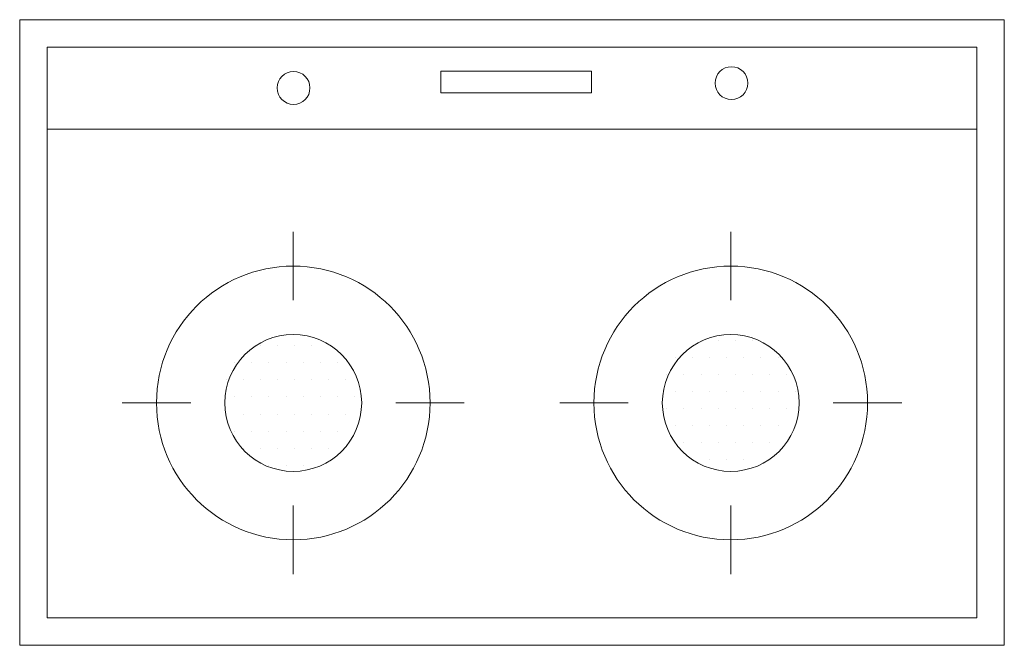
# Model space of a CAD drawing. Units: inches. Extents: x 205 to 1667, y -23 to 828.
# Tile 10 of 10: x 1560 to 1667, y 401 to 469. Entities that reach past the tile are written whole.
import ezdxf

# ---------------------------------------------------------------- set-up
doc = ezdxf.new("R2010")
doc.units = ezdxf.units.IN
doc.header["$MEASUREMENT"] = 0
doc.layers.add('A-EQPM', color=8, linetype='Continuous', lineweight=18)

# ---------------------------------------------------------------- blocks, each defined once
blk = doc.blocks.new('A$C475E21CF')
for p, q in [((0, 444.49), (0, 0)), ((0, 444.49), (699.92, 444.49)), ((699.92, 444.49), (699.92, 0)), ((19.45, 425.05), (19.45, 19.45)), ((19.45, 425.05), (680.48, 425.05)), ((680.48, 425.05), (680.48, 19.45)), ((194.48, 393.86), (194.48, 345.24)), ((505.44, 393.86), (505.44, 345.24)), ((498.43, 316.63), (498.43, 316.63)), ((510.58, 316.63), (510.58, 316.63)), ((522.74, 316.63), (522.74, 316.63)), ((185.17, 312.7), (185.17, 312.7)), ((197.32, 312.7), (197.32, 312.7)), ((209.48, 312.7), (209.48, 312.7)), ((480.19, 304.48), (480.19, 304.48)), ((492.35, 304.48), (492.35, 304.48)), ((504.5, 304.48), (504.5, 304.48)), ((516.66, 304.48), (516.66, 304.48)), ((528.81, 304.48), (528.81, 304.48)), ((540.97, 304.48), (540.97, 304.48)), ((166.94, 300.55), (166.94, 300.55)), ((179.09, 300.55), (179.09, 300.55)), ((191.25, 300.55), (191.25, 300.55)), ((203.4, 300.55), (203.4, 300.55)), ((215.56, 300.55), (215.56, 300.55)), ((227.71, 300.55), (227.71, 300.55)), ((160.86, 288.39), (160.86, 288.39)), ((173.01, 288.39), (173.01, 288.39)), ((185.17, 288.39), (185.17, 288.39)), ((197.32, 288.39), (197.32, 288.39)), ((209.48, 288.39), (209.48, 288.39)), ((221.63, 288.39), (221.63, 288.39)), ((233.79, 288.39), (233.79, 288.39)), ((474.12, 292.32), (474.12, 292.32)), ((486.27, 292.32), (486.27, 292.32)), ((498.43, 292.32), (498.43, 292.32)), ((510.58, 292.32), (510.58, 292.32)), ((522.74, 292.32), (522.74, 292.32)), ((534.89, 292.32), (534.89, 292.32)), ((547.05, 292.32), (547.05, 292.32)), ((468.04, 280.17), (468.04, 280.17)), ((480.19, 280.17), (480.19, 280.17)), ((492.35, 280.17), (492.35, 280.17)), ((504.5, 280.17), (504.5, 280.17)), ((516.66, 280.17), (516.66, 280.17)), ((528.81, 280.17), (528.81, 280.17)), ((540.97, 280.17), (540.97, 280.17)), ((553.12, 280.17), (553.12, 280.17)), ((154.78, 276.24), (154.78, 276.24)), ((166.94, 276.24), (166.94, 276.24)), ((179.09, 276.24), (179.09, 276.24)), ((191.25, 276.24), (191.25, 276.24)), ((203.4, 276.24), (203.4, 276.24)), ((215.56, 276.24), (215.56, 276.24)), ((227.71, 276.24), (227.71, 276.24)), ((239.87, 276.24), (239.87, 276.24)), ((72.93, 272.31), (121.55, 272.31)), ((267.41, 272.31), (316.03, 272.31)), ((383.89, 272.31), (432.51, 272.31)), ((461.96, 268.01), (461.96, 268.01)), ((474.12, 268.01), (474.12, 268.01)), ((486.27, 268.01), (486.27, 268.01)), ((498.43, 268.01), (498.43, 268.01)), ((510.58, 268.01), (510.58, 268.01)), ((522.74, 268.01), (522.74, 268.01)), ((534.89, 268.01), (534.89, 268.01)), ((547.05, 268.01), (547.05, 268.01)), ((578.37, 272.31), (626.99, 272.31)), ((148.7, 264.08), (148.7, 264.08)), ((160.86, 264.08), (160.86, 264.08)), ((173.01, 264.08), (173.01, 264.08)), ((185.17, 264.08), (185.17, 264.08)), ((197.32, 264.08), (197.32, 264.08)), ((209.48, 264.08), (209.48, 264.08)), ((221.63, 264.08), (221.63, 264.08)), ((233.79, 264.08), (233.79, 264.08)), ((468.04, 255.86), (468.04, 255.86)), ((480.19, 255.86), (480.19, 255.86)), ((492.35, 255.86), (492.35, 255.86)), ((504.5, 255.86), (504.5, 255.86)), ((516.66, 255.86), (516.66, 255.86)), ((528.81, 255.86), (528.81, 255.86)), ((540.97, 255.86), (540.97, 255.86)), ((553.12, 255.86), (553.12, 255.86)), ((154.78, 251.93), (154.78, 251.93)), ((166.94, 251.93), (166.94, 251.93)), ((179.09, 251.93), (179.09, 251.93)), ((191.25, 251.93), (191.25, 251.93)), ((203.4, 251.93), (203.4, 251.93)), ((215.56, 251.93), (215.56, 251.93)), ((227.71, 251.93), (227.71, 251.93)), ((239.87, 251.93), (239.87, 251.93)), ((160.86, 239.77), (160.86, 239.77)), ((173.01, 239.77), (173.01, 239.77)), ((185.17, 239.77), (185.17, 239.77)), ((197.32, 239.77), (197.32, 239.77)), ((209.48, 239.77), (209.48, 239.77)), ((221.63, 239.77), (221.63, 239.77)), ((233.79, 239.77), (233.79, 239.77)), ((474.12, 243.7), (474.12, 243.7)), ((486.27, 243.7), (486.27, 243.7)), ((498.43, 243.7), (498.43, 243.7)), ((510.58, 243.7), (510.58, 243.7)), ((522.74, 243.7), (522.74, 243.7)), ((534.89, 243.7), (534.89, 243.7)), ((547.05, 243.7), (547.05, 243.7)), ((492.35, 231.55), (492.35, 231.55)), ((504.5, 231.55), (504.5, 231.55)), ((516.66, 231.55), (516.66, 231.55)), ((528.81, 231.55), (528.81, 231.55)), ((179.09, 227.62), (179.09, 227.62)), ((191.25, 227.62), (191.25, 227.62)), ((203.4, 227.62), (203.4, 227.62)), ((215.56, 227.62), (215.56, 227.62)), ((194.48, 199.38), (194.48, 150.76)), ((505.44, 199.38), (505.44, 150.76)), ((19.45, 77.79), (680.48, 77.79)), ((293.4, 51.92), (400.62, 51.92)), ((293.4, 36.49), (293.4, 51.92)), ((400.62, 51.92), (400.62, 36.49)), ((400.62, 36.49), (293.4, 36.49)), ((19.45, 19.45), (680.48, 19.45)), ((0, 0), (699.92, 0))]:
    blk.add_line(p, q)
for centre, radius in [((194.48, 272.31), 97.24), ((505.44, 272.31), 97.24), ((194.48, 272.31), 48.62), ((505.44, 272.31), 48.62), ((193.94, 45.06), 11.67), ((505.24, 48.49), 11.67)]:
    blk.add_circle(centre, radius)
blk = doc.blocks.new('A$C1A936BB7')
blk.add_blockref('A$C475E21CF', (0, 0))

msp = doc.modelspace()

# ---------------------------------------------------------------- block references
at = {"layer": 'A-EQPM', "xscale": 0.1533552163418108, "yscale": 0.1533552163418108, "zscale": 0.1533552163418108, "rotation": 180}
msp.add_blockref('A$C1A936BB7', (1666.8668, 468.9999), dxfattribs=at)

doc.saveas('drawing.dxf')
